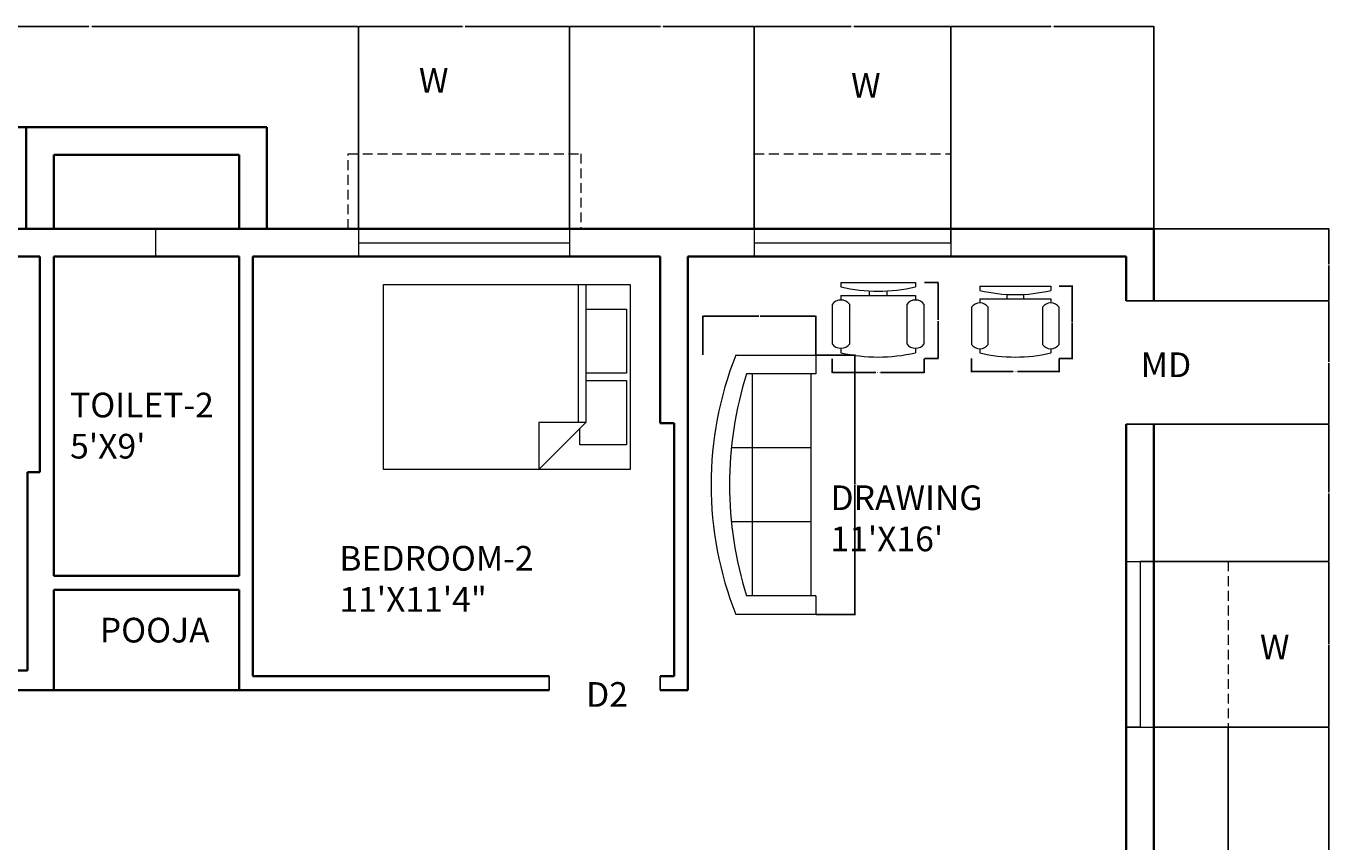
# Model space of a CAD drawing. Units: inches. Extents: x 514 to 1200, y -110 to 470.
# Tile 3 of 3: x 777 to 1200, y 206 to 470. Entities that reach past the tile are written whole.
import ezdxf

# ---------------------------------------------------------------- set-up
doc = ezdxf.new("R2010")
doc.units = ezdxf.units.IN
doc.linetypes.add('HIDDEN2', pattern=[4.7625, 3.175, -1.5875])
for name, color, linetype, lineweight in [('A-ANNO-DIMS', 2, 'Continuous', 18), ('A-ANNO-IDEN', 3, 'Continuous', 18), ('A-AREA-IDEN', 7, 'Continuous', 18), ('A-DOOR', 3, 'Continuous', 25), ('A-FLOR-OVHD', 8, 'HIDDEN2', 18), ('A-FURN', 8, 'Continuous', 18), ('A-GLAZ', 4, 'Continuous', 18), ('A-WALL', 7, 'Continuous', 35)]:
    doc.layers.add(name, color=color, linetype=linetype, lineweight=lineweight)
doc.dimstyles.get("Standard").update_dxf_attribs({"dimtxt": 0.18, "dimasz": 0.18, "dimexe": 0.18, "dimexo": 0.0625, "dimgap": 0.09, "dimtad": 0, "dimtih": 1, "dimtoh": 1, "dimdec": 4, "dimzin": 0, "dimdsep": 46, "dimtxsty": 'Standard', "dimcen": 0.09, "dimadec": 0, "dimazin": 0, "dimtfac": 1, "dimtdec": 4, "dimtofl": 0, "dimtmove": 0, "dimatfit": 3, "dimfxl": 1, "dimtolj": 1, "dimtzin": 0, "dimarcsym": 0})

# ---------------------------------------------------------------- blocks, each defined once
blk = doc.blocks.new('Chair - Desk')
for p, q in [((-8.5, 0), (-8.5, -1)), ((-8.5, 0), (8.5, 0)), ((8.5, 0), (8.5, -1)), ((-2, -3), (-2, -1.9355)), ((2, -1.9576), (2, -3)), ((-10.5, -5), (-10.5, -14)), ((-8.5, -3), (-8.5, -4)), ((-8.5, -3), (8.5, -3)), ((-6.5, -14), (-6.5, -5)), ((6.5, -5), (6.5, -14)), ((8.5, -3), (8.5, -4)), ((10.5, -14), (10.5, -5)), ((-8.5, -15), (-8.5, -16)), ((8.5, -15), (8.5, -16))]:
    blk.add_line(p, q)
for centre, radius, start, end in [((0, 34.625), 36.625, 256.5803, 283.4197), ((-8.5, -6.5), 2.5, 36.8699, 143.1301), ((8.5, -6.5), 2.5, 36.8699, 143.1301), ((-8.5, -12.5), 2.5, 216.8699, 323.1301), ((8.5, -12.5), 2.5, 216.8699, 323.1301), ((0, 19.625), 36.625, 256.5803, 283.4197)]:
    blk.add_arc(centre, radius, start, end)
blk = doc.blocks.new('Sofa - Roundback 7 ft.')
for p, q in [((-12.00002, -32.4421), (-12.00003, -6.5971)), ((11.99997, -32.4421), (11.99998, -6.5971)), ((-36.000027, -34), (-36.000027, -11.4696)), ((35.99998, -34), (35.99998, -11.4696)), ((-35.999844, -13.3819), (35.9998, -13.3819)), ((-36.000027, -32.4421), (35.99998, -32.4421))]:
    blk.add_line(p, q)
for points in [[(-36.000027, -34), (-42.000027, -34), (-42.000027, -8)], [(41.99998, -8), (41.99998, -34), (35.99998, -34)]]:
    blk.add_lwpolyline(points)
for centre, radius, start, end in [((0, -114.25), 114.25, 68.43141, 111.5686), ((-0.00001, -127.1968), 121.1968, 72.72033, 107.2797)]:
    blk.add_arc(centre, radius, start, end)
blk = doc.blocks.new('Bed - Queen')
for p, q in [((0, -80.00003), (0, 0)), ((0, 0), (59.99999, 0)), ((59.99999, 0), (59.99999, -80.00003)), ((7.99999, -1.2), (28.79998, -1.2)), ((7.99999, -14.4), (7.99999, -1.2)), ((28.79998, -1.2), (28.79998, -14.4)), ((31.19999, -1.2), (51.99999, -1.2)), ((31.19999, -14.4), (31.19999, -1.2)), ((51.99999, -1.2), (51.99999, -16.4)), ((0, -14.4), (44.8, -14.4)), ((44.8, -16.8), (0, -16.8)), ((59.99999, -29.6), (44.8, -14.4)), ((44.8, -14.4), (44.8, -29.6)), ((51.99999, -16.4), (46.79936, -16.4)), ((44.8, -29.6), (59.99999, -29.6)), ((59.99999, -80.00003), (0, -80.00003))]:
    blk.add_line(p, q)
blk = doc.blocks.new('WALL-BAY-60x24')
for p, q in [((0, 33), (0, 0)), ((9, 33), (9, 9)), ((69, 9), (69, 33)), ((78, 0), (78, 33)), ((9, 9), (69, 9)), ((0, 0), (78, 0))]:
    blk.add_line(p, q)
blk = doc.blocks.new('*D8')
at = {"layer": 'A-ANNO-DIMS', "color": 0, "lineweight": -2, "transparency": 16777216}
for p, q in [((1083.8, 362.46), (1083.8, 358.09)), ((1112.14, 362.46), (1112.14, 358.09)), ((1083.98, 358.27), (1097.22, 358.27)), ((1111.96, 358.27), (1098.72, 358.27))]:
    blk.add_line(p, q, dxfattribs=at)
at = {"layer": 'A-ANNO-DIMS', "color": 0, "transparency": 16777216}
for points in [[(1083.98, 358.3), (1083.98, 358.24), (1083.8, 358.27)], [(1111.96, 358.3), (1111.96, 358.24), (1112.14, 358.27)]]:
    blk.add_solid(points, dxfattribs=at)
at = {"layer": 'Defpoints', "color": 0, "transparency": 16777216}
for p in [(1083.8, 362.52), (1112.14, 362.52), (1112.14, 358.27)]:
    blk.add_point(p, dxfattribs=at)
at = {"layer": 'A-ANNO-DIMS', "color": 0, "transparency": 16777216, "insert": (1097.97, 358.27), "char_height": 0.18, "attachment_point": 5}
blk.add_mtext('\\A1;CHAIR 28', dxfattribs=at)
blk = doc.blocks.new('*D9')
at = {"layer": 'A-ANNO-DIMS', "color": 0, "lineweight": -2, "transparency": 16777216}
for p, q in [((1112.2, 385.91), (1116.57, 385.91)), ((1116.39, 385.73), (1116.39, 374.4)), ((1116.39, 362.7), (1116.39, 374.04)), ((1112.2, 362.52), (1116.57, 362.52))]:
    blk.add_line(p, q, dxfattribs=at)
at = {"layer": 'A-ANNO-DIMS', "color": 0, "transparency": 16777216}
for points in [[(1116.36, 385.73), (1116.42, 385.73), (1116.39, 385.91)], [(1116.36, 362.7), (1116.42, 362.7), (1116.39, 362.52)]]:
    blk.add_solid(points, dxfattribs=at)
at = {"layer": 'Defpoints', "color": 0, "transparency": 16777216}
for p in [(1112.14, 385.91), (1116.39, 385.91), (1112.14, 362.52)]:
    blk.add_point(p, dxfattribs=at)
at = {"layer": 'A-ANNO-DIMS', "color": 0, "transparency": 16777216, "insert": (1116.39, 374.22), "char_height": 0.18, "attachment_point": 5}
blk.add_mtext('\\A1;23', dxfattribs=at)
blk = doc.blocks.new('*D12')
at = {"layer": 'A-ANNO-DIMS', "color": 0, "lineweight": -2, "transparency": 16777216}
for p, q in [((1038.59, 362.44), (1038.59, 357.84)), ((1068.46, 362.44), (1068.46, 357.84)), ((1038.77, 358.02), (1052.79, 358.02)), ((1068.28, 358.02), (1054.26, 358.02))]:
    blk.add_line(p, q, dxfattribs=at)
at = {"layer": 'A-ANNO-DIMS', "color": 0, "transparency": 16777216}
for points in [[(1038.77, 358.05), (1038.77, 357.99), (1038.59, 358.02)], [(1068.28, 358.05), (1068.28, 357.99), (1068.46, 358.02)]]:
    blk.add_solid(points, dxfattribs=at)
at = {"layer": 'Defpoints', "color": 0, "transparency": 16777216}
for p in [(1038.59, 362.5), (1068.46, 362.5), (1068.46, 358.02)]:
    blk.add_point(p, dxfattribs=at)
at = {"layer": 'A-ANNO-DIMS', "color": 0, "transparency": 16777216, "insert": (1053.53, 358.02), "char_height": 0.18, "attachment_point": 5}
blk.add_mtext('\\A1;CHAIR 30', dxfattribs=at)
blk = doc.blocks.new('*D13')
at = {"layer": 'A-ANNO-DIMS', "color": 0, "lineweight": -2, "transparency": 16777216}
for p, q in [((1068.52, 387.15), (1073.12, 387.15)), ((1072.94, 386.97), (1072.94, 375.01)), ((1072.94, 362.68), (1072.94, 374.65)), ((1068.52, 362.5), (1073.12, 362.5))]:
    blk.add_line(p, q, dxfattribs=at)
at = {"layer": 'A-ANNO-DIMS', "color": 0, "transparency": 16777216}
for points in [[(1072.91, 386.97), (1072.97, 386.97), (1072.94, 387.15)], [(1072.91, 362.68), (1072.97, 362.68), (1072.94, 362.5)]]:
    blk.add_solid(points, dxfattribs=at)
at = {"layer": 'Defpoints', "color": 0, "transparency": 16777216}
for p in [(1068.46, 387.15), (1072.94, 387.15), (1068.46, 362.5)]:
    blk.add_point(p, dxfattribs=at)
at = {"layer": 'A-ANNO-DIMS', "color": 0, "transparency": 16777216, "insert": (1072.94, 374.83), "char_height": 0.18, "attachment_point": 5}
blk.add_mtext('\\A1;25', dxfattribs=at)
blk = doc.blocks.new('*D18')
at = {"layer": 'A-ANNO-DIMS', "color": 0, "lineweight": -2, "transparency": 16777216}
for p, q in [((1033.43, 363.59), (1046.15, 363.59)), ((1045.97, 363.41), (1045.97, 321.77)), ((1045.97, 279.77), (1045.97, 321.41)), ((1033.43, 279.59), (1046.15, 279.59))]:
    blk.add_line(p, q, dxfattribs=at)
at = {"layer": 'A-ANNO-DIMS', "color": 0, "transparency": 16777216}
for points in [[(1045.94, 363.41), (1046, 363.41), (1045.97, 363.59)], [(1045.94, 279.77), (1046, 279.77), (1045.97, 279.59)]]:
    blk.add_solid(points, dxfattribs=at)
at = {"layer": 'Defpoints', "color": 0, "transparency": 16777216}
for p in [(1033.37, 363.59), (1045.97, 363.59), (1033.37, 279.59)]:
    blk.add_point(p, dxfattribs=at)
at = {"layer": 'A-ANNO-DIMS', "color": 0, "transparency": 16777216, "insert": (1045.97, 321.59), "char_height": 0.18, "attachment_point": 5}
blk.add_mtext('\\A1;SOFA 84', dxfattribs=at)
blk = doc.blocks.new('*D19')
at = {"layer": 'A-ANNO-DIMS', "color": 0, "lineweight": -2, "transparency": 16777216}
for p, q in [((996.7, 363.65), (996.7, 376.37)), ((996.88, 376.19), (1014.8, 376.19)), ((1033.19, 376.19), (1015.28, 376.19)), ((1033.37, 363.65), (1033.37, 376.37))]:
    blk.add_line(p, q, dxfattribs=at)
at = {"layer": 'A-ANNO-DIMS', "color": 0, "transparency": 16777216}
for points in [[(996.88, 376.22), (996.88, 376.16), (996.7, 376.19)], [(1033.19, 376.22), (1033.19, 376.16), (1033.37, 376.19)]]:
    blk.add_solid(points, dxfattribs=at)
at = {"layer": 'Defpoints', "color": 0, "transparency": 16777216}
for p in [(996.7, 376.19), (996.7, 363.59), (1033.37, 363.59)]:
    blk.add_point(p, dxfattribs=at)
at = {"layer": 'A-ANNO-DIMS', "color": 0, "transparency": 16777216, "insert": (1015.04, 376.19), "char_height": 0.18, "attachment_point": 5}
blk.add_mtext('\\A1;37', dxfattribs=at)
blk = doc.blocks.new('*D26')
at = {"layer": 'A-ANNO-DIMS', "color": 0, "lineweight": -2, "transparency": 16777216}
for p, q in [((711.28, 404.58), (711.28, 470.25)), ((711.46, 470.07), (797.69, 470.07)), ((884.94, 470.07), (798.71, 470.07)), ((885.12, 404.58), (885.12, 470.25))]:
    blk.add_line(p, q, dxfattribs=at)
at = {"layer": 'A-ANNO-DIMS', "color": 0, "transparency": 16777216}
for points in [[(711.46, 470.1), (711.46, 470.04), (711.28, 470.07)], [(884.94, 470.1), (884.94, 470.04), (885.12, 470.07)]]:
    blk.add_solid(points, dxfattribs=at)
at = {"layer": 'Defpoints', "color": 0, "transparency": 16777216}
for p in [(885.12, 470.07), (711.28, 404.52), (885.12, 404.52)]:
    blk.add_point(p, dxfattribs=at)
at = {"layer": 'A-ANNO-DIMS', "color": 0, "transparency": 16777216, "insert": (798.2, 470.07), "char_height": 0.18, "attachment_point": 5}
blk.add_mtext('\\A1;173.83', dxfattribs=at)
blk = doc.blocks.new('*D27')
at = {"layer": 'A-ANNO-DIMS', "color": 0, "lineweight": -2, "transparency": 16777216}
for p, q in [((885.12, 404.58), (885.12, 470.25)), ((885.3, 470.07), (918.83, 470.07)), ((953.26, 470.07), (919.73, 470.07)), ((953.44, 404.58), (953.44, 470.25))]:
    blk.add_line(p, q, dxfattribs=at)
at = {"layer": 'A-ANNO-DIMS', "color": 0, "transparency": 16777216}
for points in [[(885.3, 470.1), (885.3, 470.04), (885.12, 470.07)], [(953.26, 470.1), (953.26, 470.04), (953.44, 470.07)]]:
    blk.add_solid(points, dxfattribs=at)
at = {"layer": 'Defpoints', "color": 0, "transparency": 16777216}
for p in [(953.44, 470.07), (885.12, 404.52), (953.44, 404.52)]:
    blk.add_point(p, dxfattribs=at)
at = {"layer": 'A-ANNO-DIMS', "color": 0, "transparency": 16777216, "insert": (919.28, 470.07), "char_height": 0.18, "attachment_point": 5}
blk.add_mtext('\\A1;68.32', dxfattribs=at)
blk = doc.blocks.new('*D28')
at = {"layer": 'A-ANNO-DIMS', "color": 0, "lineweight": -2, "transparency": 16777216}
for p, q in [((953.44, 404.58), (953.44, 470.25)), ((953.62, 470.07), (982.96, 470.07)), ((1013.2, 470.07), (983.86, 470.07)), ((1013.38, 404.58), (1013.38, 470.25))]:
    blk.add_line(p, q, dxfattribs=at)
at = {"layer": 'A-ANNO-DIMS', "color": 0, "transparency": 16777216}
for points in [[(953.62, 470.1), (953.62, 470.04), (953.44, 470.07)], [(1013.2, 470.1), (1013.2, 470.04), (1013.38, 470.07)]]:
    blk.add_solid(points, dxfattribs=at)
at = {"layer": 'Defpoints', "color": 0, "transparency": 16777216}
for p in [(1013.38, 470.07), (953.44, 404.52), (1013.38, 404.52)]:
    blk.add_point(p, dxfattribs=at)
at = {"layer": 'A-ANNO-DIMS', "color": 0, "transparency": 16777216, "insert": (983.41, 470.07), "char_height": 0.18, "attachment_point": 5}
blk.add_mtext('\\A1;59.94', dxfattribs=at)
blk = doc.blocks.new('*D29')
at = {"layer": 'A-ANNO-DIMS', "color": 0, "lineweight": -2, "transparency": 16777216}
for p, q in [((1013.377732, 404.583196), (1013.377732, 470.250696)), ((1013.557732, 470.070696), (1044.750738, 470.070696)), ((1076.843744, 470.070696), (1045.650738, 470.070696)), ((1077.023744, 404.583196), (1077.023744, 470.250696))]:
    blk.add_line(p, q, dxfattribs=at)
at = {"layer": 'A-ANNO-DIMS', "color": 0, "transparency": 16777216}
for points in [[(1013.557732, 470.100696), (1013.557732, 470.040696), (1013.377732, 470.070696)], [(1076.843744, 470.100696), (1076.843744, 470.040696), (1077.023744, 470.070696)]]:
    blk.add_solid(points, dxfattribs=at)
at = {"layer": 'Defpoints', "color": 0, "transparency": 16777216}
for p in [(1077.023744, 470.070696), (1013.377732, 404.520696), (1077.023744, 404.520696)]:
    blk.add_point(p, dxfattribs=at)
at = {"layer": 'A-ANNO-DIMS', "color": 0, "transparency": 16777216, "insert": (1045.200738, 470.070696), "char_height": 0.18, "attachment_point": 5}
blk.add_mtext('\\A1;63.65', dxfattribs=at)
blk = doc.blocks.new('*D30')
at = {"layer": 'A-ANNO-DIMS', "color": 0, "lineweight": -2, "transparency": 16777216}
for p, q in [((1077.023744, 404.583196), (1077.023744, 470.250696)), ((1077.203744, 470.070696), (1109.507154, 470.070696)), ((1142.710564, 470.070696), (1110.407154, 470.070696)), ((1142.890564, 404.583196), (1142.890564, 470.250696))]:
    blk.add_line(p, q, dxfattribs=at)
at = {"layer": 'A-ANNO-DIMS', "color": 0, "transparency": 16777216}
for points in [[(1077.203744, 470.100696), (1077.203744, 470.040696), (1077.023744, 470.070696)], [(1142.710564, 470.100696), (1142.710564, 470.040696), (1142.890564, 470.070696)]]:
    blk.add_solid(points, dxfattribs=at)
at = {"layer": 'Defpoints', "color": 0, "transparency": 16777216}
for p in [(1142.890564, 470.070696), (1077.023744, 404.520696), (1142.890564, 404.520696)]:
    blk.add_point(p, dxfattribs=at)
at = {"layer": 'A-ANNO-DIMS', "color": 0, "transparency": 16777216, "insert": (1109.957154, 470.070696), "char_height": 0.18, "attachment_point": 5}
blk.add_mtext('\\A1;65.87', dxfattribs=at)
blk = doc.blocks.new('*D31')
at = {"layer": 'A-ANNO-DIMS', "color": 0, "lineweight": -2, "transparency": 16777216}
for p, q in [((1142.953064, 404.520696), (1199.719295, 404.520696)), ((1199.539295, 404.340696), (1199.539295, 393.046922)), ((1199.539295, 381.393148), (1199.539295, 392.686922)), ((1142.953064, 381.213148), (1199.719295, 381.213148))]:
    blk.add_line(p, q, dxfattribs=at)
at = {"layer": 'A-ANNO-DIMS', "color": 0, "transparency": 16777216}
for points in [[(1199.509295, 404.340696), (1199.569295, 404.340696), (1199.539295, 404.520696)], [(1199.509295, 381.393148), (1199.569295, 381.393148), (1199.539295, 381.213148)]]:
    blk.add_solid(points, dxfattribs=at)
at = {"layer": 'Defpoints', "color": 0, "transparency": 16777216}
for p in [(1142.890564, 404.520696), (1142.890564, 381.213148), (1199.539295, 381.213148)]:
    blk.add_point(p, dxfattribs=at)
at = {"layer": 'A-ANNO-DIMS', "color": 0, "transparency": 16777216, "insert": (1199.539295, 392.866922), "char_height": 0.18, "attachment_point": 5}
blk.add_mtext('\\A1;23.308', dxfattribs=at)
blk = doc.blocks.new('*D32')
at = {"layer": 'A-ANNO-DIMS', "color": 0, "lineweight": -2, "transparency": 16777216}
for p, q in [((1142.953064, 381.213148), (1199.719295, 381.213148)), ((1199.539295, 381.033148), (1199.539295, 361.393148)), ((1199.539295, 341.393148), (1199.539295, 361.033148)), ((1142.953064, 341.213148), (1199.719295, 341.213148))]:
    blk.add_line(p, q, dxfattribs=at)
at = {"layer": 'A-ANNO-DIMS', "color": 0, "transparency": 16777216}
for points in [[(1199.509295, 381.033148), (1199.569295, 381.033148), (1199.539295, 381.213148)], [(1199.509295, 341.393148), (1199.569295, 341.393148), (1199.539295, 341.213148)]]:
    blk.add_solid(points, dxfattribs=at)
at = {"layer": 'Defpoints', "color": 0, "transparency": 16777216}
for p in [(1142.890564, 381.213148), (1142.890564, 341.213148), (1199.539295, 341.213148)]:
    blk.add_point(p, dxfattribs=at)
at = {"layer": 'A-ANNO-DIMS', "color": 0, "transparency": 16777216, "insert": (1199.539295, 361.213148), "char_height": 0.18, "attachment_point": 5}
blk.add_mtext('\\A1;40', dxfattribs=at)
blk = doc.blocks.new('*D33')
at = {"layer": 'A-ANNO-DIMS', "color": 0, "lineweight": -2, "transparency": 16777216}
for p, q in [((1142.953064, 341.213148), (1199.719295, 341.213148)), ((1199.539295, 341.033148), (1199.539295, 319.140993)), ((1199.539295, 296.888838), (1199.539295, 318.780993)), ((1142.953064, 296.708838), (1199.719295, 296.708838))]:
    blk.add_line(p, q, dxfattribs=at)
at = {"layer": 'A-ANNO-DIMS', "color": 0, "transparency": 16777216}
for points in [[(1199.509295, 341.033148), (1199.569295, 341.033148), (1199.539295, 341.213148)], [(1199.509295, 296.888838), (1199.569295, 296.888838), (1199.539295, 296.708838)]]:
    blk.add_solid(points, dxfattribs=at)
at = {"layer": 'Defpoints', "color": 0, "transparency": 16777216}
for p in [(1142.890564, 341.213148), (1142.890564, 296.708838), (1199.539295, 296.708838)]:
    blk.add_point(p, dxfattribs=at)
at = {"layer": 'A-ANNO-DIMS', "color": 0, "transparency": 16777216, "insert": (1199.539295, 318.960993), "char_height": 0.18, "attachment_point": 5}
blk.add_mtext('\\A1;44.5', dxfattribs=at)
blk = doc.blocks.new('*D34')
at = {"layer": 'A-ANNO-DIMS', "color": 0, "lineweight": -2, "transparency": 16777216}
for p, q in [((1142.953064, 296.708838), (1199.719295, 296.708838)), ((1199.539295, 296.528838), (1199.539295, 270.069776)), ((1199.539295, 243.250714), (1199.539295, 269.709776)), ((1142.953064, 243.070714), (1199.719295, 243.070714))]:
    blk.add_line(p, q, dxfattribs=at)
at = {"layer": 'A-ANNO-DIMS', "color": 0, "transparency": 16777216}
for points in [[(1199.509295, 296.528838), (1199.569295, 296.528838), (1199.539295, 296.708838)], [(1199.509295, 243.250714), (1199.569295, 243.250714), (1199.539295, 243.070714)]]:
    blk.add_solid(points, dxfattribs=at)
at = {"layer": 'Defpoints', "color": 0, "transparency": 16777216}
for p in [(1142.890564, 296.708838), (1142.890564, 243.070714), (1199.539295, 243.070714)]:
    blk.add_point(p, dxfattribs=at)
at = {"layer": 'A-ANNO-DIMS', "color": 0, "transparency": 16777216, "insert": (1199.539295, 269.889776), "char_height": 0.18, "attachment_point": 5}
blk.add_mtext('\\A1;53.64', dxfattribs=at)
blk = doc.blocks.new('*D35')
at = {"layer": 'A-ANNO-DIMS', "color": 0, "lineweight": -2, "transparency": 16777216}
for p, q in [((1142.953064, 243.070714), (1199.719295, 243.070714)), ((1199.539295, 242.890714), (1199.539295, 136.225705)), ((1199.539295, 29.200696), (1199.539295, 135.865705)), ((1142.953064, 29.020696), (1199.719295, 29.020696))]:
    blk.add_line(p, q, dxfattribs=at)
at = {"layer": 'A-ANNO-DIMS', "color": 0, "transparency": 16777216}
for points in [[(1199.509295, 242.890714), (1199.569295, 242.890714), (1199.539295, 243.070714)], [(1199.509295, 29.200696), (1199.569295, 29.200696), (1199.539295, 29.020696)]]:
    blk.add_solid(points, dxfattribs=at)
at = {"layer": 'Defpoints', "color": 0, "transparency": 16777216}
for p in [(1142.890564, 243.070714), (1142.890564, 29.020696), (1199.539295, 29.020696)]:
    blk.add_point(p, dxfattribs=at)
at = {"layer": 'A-ANNO-DIMS', "color": 0, "transparency": 16777216, "insert": (1199.539295, 136.045705), "char_height": 0.18, "attachment_point": 5}
blk.add_mtext('\\A1;214.05', dxfattribs=at)
blk = doc.blocks.new('*D36')
at = {"layer": 'A-ANNO-DIMS', "color": 0, "lineweight": -2, "transparency": 16777216}
for p, q in [((1166.99, 243.01), (1166.99, -83.71)), ((547.32, 185.96), (547.32, -83.71)), ((547.5, -83.53), (856.73, -83.53)), ((1166.81, -83.53), (857.57, -83.53))]:
    blk.add_line(p, q, dxfattribs=at)
at = {"layer": 'A-ANNO-DIMS', "color": 0, "transparency": 16777216}
for points in [[(547.5, -83.5), (547.5, -83.56), (547.32, -83.53)], [(1166.81, -83.5), (1166.81, -83.56), (1166.99, -83.53)]]:
    blk.add_solid(points, dxfattribs=at)
at = {"layer": 'Defpoints', "color": 0, "transparency": 16777216}
for p in [(1166.99, 243.07), (547.32, 186.02), (1166.99, -83.53)]:
    blk.add_point(p, dxfattribs=at)
at = {"layer": 'A-ANNO-DIMS', "color": 0, "transparency": 16777216, "insert": (857.15, -83.53), "char_height": 0.18, "attachment_point": 5}
blk.add_mtext('\\A1;619.7', dxfattribs=at)
blk = doc.blocks.new('*D37')
at = {"layer": 'A-ANNO-DIMS', "color": 0, "lineweight": -2, "transparency": 16777216}
for p, q in [((719.82324, 437.520696), (514.588716, 437.520696)), ((514.768716, 437.340696), (514.768716, 193.450696)), ((514.768716, -50.799304), (514.768716, 193.090696)), ((846.828064, -50.979304), (514.588716, -50.979304))]:
    blk.add_line(p, q, dxfattribs=at)
at = {"layer": 'A-ANNO-DIMS', "color": 0, "transparency": 16777216}
for points in [[(514.738716, 437.340696), (514.798716, 437.340696), (514.768716, 437.520696)], [(514.738716, -50.799304), (514.798716, -50.799304), (514.768716, -50.979304)]]:
    blk.add_solid(points, dxfattribs=at)
at = {"layer": 'Defpoints', "color": 0, "transparency": 16777216}
for p in [(514.768716, 437.520696), (719.88574, 437.520696), (846.890564, -50.979304)]:
    blk.add_point(p, dxfattribs=at)
at = {"layer": 'A-ANNO-DIMS', "color": 0, "transparency": 16777216, "insert": (514.768716, 193.270696), "char_height": 0.18, "attachment_point": 5}
blk.add_mtext('\\A1;488.5', dxfattribs=at)

msp = doc.modelspace()

# ---------------------------------------------------------------- linework, layer by layer
at = {"layer": 'A-DOOR'}
for p, q in [((1133.8906, 381.2131), (1142.8906, 381.2131)), ((1142.8906, 341.2131), (1133.8906, 341.2131)), ((1138.3906, 341.2131), (1142.8906, 341.2131)), ((946.8906, 255.0207), (946.8906, 259.5207)), ((982.8906, 255.0207), (982.8906, 259.5207))]:
    msp.add_line(p, q, dxfattribs=at)
at = {"layer": 'A-FLOR-OVHD'}
for p, q in [((881.7608, 404.5207), (881.7608, 428.8855)), ((881.7608, 428.8855), (957.1619, 428.8855)), ((957.1619, 428.8855), (957.1619, 404.5207)), ((1013.3777, 404.5207), (1013.3777, 428.8855)), ((1013.3777, 428.8855), (1077.0237, 428.8855)), ((1077.0237, 428.8855), (1077.0237, 404.5207)), ((1142.8906, 296.7088), (1166.9893, 296.7088)), ((1166.9893, 296.7088), (1166.9893, 243.0707)), ((1166.9893, 243.0707), (1142.8906, 243.0707))]:
    msp.add_line(p, q, dxfattribs=at)
at = {"layer": 'A-GLAZ'}
for p, q in [((819.3159, 404.5207), (819.3159, 395.5207)), ((885.1179, 404.5207), (885.1179, 395.5207)), ((953.4385, 404.5207), (953.4385, 395.5207)), ((1013.3777, 404.5207), (1013.3777, 395.5207)), ((1077.0237, 404.5207), (1077.0237, 395.5207)), ((1077.0237, 400.0207), (1077.0237, 404.5207)), ((1077.0237, 404.5207), (1077.0237, 395.5207)), ((885.1179, 400.0207), (953.4385, 400.0207)), ((1013.3777, 400.0207), (1077.0237, 400.0207)), ((1133.8906, 296.7088), (1142.8906, 296.7088)), ((1142.8906, 296.7088), (1138.3906, 296.7088)), ((1138.3906, 296.7088), (1138.3906, 243.0707)), ((1138.3906, 243.0707), (1133.8906, 243.0707)), ((1133.8906, 243.0707), (1142.8906, 243.0707))]:
    msp.add_line(p, q, dxfattribs=at)
at = {"layer": 'A-WALL'}
for p, q in [((777.3906, 437.5207), (728.8857, 437.5207)), ((728.8857, 404.5207), (1142.8906, 404.5207)), ((1142.8906, 395.5207), (1142.8906, 404.5207)), ((609.8906, 395.5207), (781.8906, 395.5207)), ((781.8906, 325.6278), (781.8906, 395.5207)), ((786.3906, 292.0207), (786.3906, 395.5207)), ((786.3906, 395.5207), (846.3906, 395.5207)), ((846.3906, 292.0207), (846.3906, 395.5207)), ((850.8906, 259.5207), (850.8906, 395.5207)), ((850.8906, 395.5207), (982.8906, 395.5207)), ((982.8906, 341.5561), (982.8906, 395.5207)), ((991.8906, 255.0207), (991.8906, 395.5207)), ((991.8906, 395.5207), (1133.8906, 395.5207)), ((1133.8906, 381.2131), (1133.8906, 395.5207)), ((1142.8906, 381.2131), (1142.8906, 395.5207)), ((982.8906, 341.5561), (987.3906, 341.5561)), ((987.3906, 259.5207), (987.3906, 341.5561)), ((1133.8906, 255.0207), (1133.8906, 341.2131)), ((1142.8906, 255.0207), (1142.8906, 341.2131)), ((777.8906, 261.4252), (777.8906, 325.6278)), ((777.8906, 325.6278), (781.8906, 325.6278)), ((786.3906, 292.0207), (846.3906, 292.0207)), ((786.3906, 255.0207), (786.3906, 287.5207)), ((786.3906, 287.5207), (846.3906, 287.5207)), ((846.3906, 255.0207), (846.3906, 287.5207)), ((772.9065, 261.4252), (777.8906, 261.4252)), ((850.8906, 259.5207), (946.8906, 259.5207)), ((987.3906, 259.5207), (982.8906, 259.5207)), ((777.8906, 255.0207), (772.9065, 255.0207)), ((777.8906, 255.0207), (786.3906, 255.0207)), ((777.8906, 255.0207), (946.8906, 255.0207)), ((786.3906, 255.0207), (846.3906, 255.0207)), ((991.8906, 255.0207), (982.8906, 255.0207)), ((1133.8906, 255.0207), (1133.8906, 199.0207)), ((1142.8906, 255.0207), (1142.8906, 199.0207))]:
    msp.add_line(p, q, dxfattribs=at)

# ---------------------------------------------------------------- block references
at = {"layer": 'A-FURN'}
for name, p, rotation in [('Bed - Queen', (973.1991, 386.5264), 270), ('Sofa - Roundback 7 ft.', (999.3688, 321.5877), 90)]:
    msp.add_blockref(name, p, dxfattribs=dict(at, rotation=rotation))
for p, xscale, yscale, zscale in [((1053.5268, 387.1502), 1.422102317285446, 1.422102317285446, 1.422102317285446), ((1097.9695, 385.9114), 1.349230775328343, 1.349230775328343, 1.349230775328343)]:
    msp.add_blockref('Chair - Desk', p, dxfattribs=dict(at, xscale=xscale, yscale=yscale, zscale=zscale))
at = {"layer": 'A-WALL', "rotation": 180}
msp.add_blockref('WALL-BAY-60x24', (855.3906, 437.5207), dxfattribs=at)

# ---------------------------------------------------------------- texts
at = {"layer": 'A-ANNO-IDEN', "char_height": 8, "attachment_point": 1}
for s, insert in [('{\\fTimes New Roman|b0|i0|c0|p18;W}', (904.6938, 456.6502)), ('{\\fTimes New Roman|b0|i0|c0|p18;W}', (1044.7366, 455.055)), ('{\\fTimes New Roman|b0|i0|c0|p18;MD}', (1138.598, 364.4832)), ('{\\fTimes New Roman|b0|i0|c0|p18;W}', (1177.2378, 273.0239)), ('{\\fTimes New Roman|b0|i0|c0|p18;D2}', (958.8675, 257.6241))]:
    msp.add_mtext_dynamic_manual_height_columns(s, width=92.773282, gutter_width=12.5, heights=[0], dxfattribs=dict(at, insert=insert))
at = {"layer": 'A-AREA-IDEN', "char_height": 8, "attachment_point": 1}
for s, insert in [("{\\fTimes New Roman|b0|i0|c0|p18;TOILET-2\\P5'X9'}", (791.661, 351.4229)), ("{\\fTimes New Roman|b0|i0|c0|p18;DRAWING\\P11'X16'}", (1038.0527, 321.3746)), ('{\\fTimes New Roman|b0|i0|c0|p18;BEDROOM-2\\P11\'X11\'4"}', (878.9146, 301.7593)), ('{\\fTimes New Roman|b0|i0|c0|p18;POOJA}', (801.2933, 278.4627))]:
    msp.add_mtext_dynamic_manual_height_columns(s, width=92.773282, gutter_width=12.5, heights=[0], dxfattribs=dict(at, insert=insert))

# ---------------------------------------------------------------- dimensions: what is measured, and where the dimension line sits
at = {"layer": 'A-ANNO-DIMS'}
for base, p1, p2, override, picture, middle in [((885.1179, 470.0707), (711.283, 404.5207), (885.1179, 404.5207), {"dimdec": 2, "dimlfac": 1, "dimrnd": 0, "dimzin": 0, "dimdsep": 46, "dimlunit": 2}, '*D26', (798.2005, 470.0707)), ((953.4385, 470.0707), (885.1179, 404.5207), (953.4385, 404.5207), {"dimdec": 2, "dimlfac": 1, "dimrnd": 0, "dimzin": 0, "dimdsep": 46, "dimlunit": 2}, '*D27', (919.2782, 470.0707)), ((1013.3777, 470.0707), (953.4385, 404.5207), (1013.3777, 404.5207), {"dimdec": 2, "dimlfac": 1, "dimrnd": 0, "dimzin": 0, "dimdsep": 46, "dimlunit": 2}, '*D28', (983.4081, 470.0707)), ((1077.0237, 470.0707), (1013.3777, 404.5207), (1077.0237, 404.5207), {"dimdec": 2, "dimlfac": 1, "dimrnd": 0, "dimzin": 0, "dimdsep": 46, "dimlunit": 2}, '*D29', (1045.2007, 470.0707)), ((1142.8906, 470.0707), (1077.0237, 404.5207), (1142.8906, 404.5207), {"dimdec": 2, "dimlfac": 1, "dimrnd": 0, "dimzin": 0, "dimdsep": 46, "dimlunit": 2}, '*D30', (1109.9572, 470.0707)), ((1166.9893, -83.5293), (547.3187, 186.0207), (1166.9893, 243.0707), {"dimdec": 1, "dimlfac": 1, "dimrnd": 0, "dimzin": 0, "dimdsep": 46, "dimlunit": 2}, '*D36', (857.154, -83.5293))]:
    dim = msp.add_linear_dim(base=base, p1=p1, p2=p2, dimstyle='Standard', override=override, dxfattribs=at)
    dim.commit()
    dim.dimension.update_dxf_attribs({"geometry": picture, "text_midpoint": middle})
for base, p1, p2, angle, override, picture, middle in [((514.7687, 437.5207), (846.8906, -50.9793), (719.8857, 437.5207), 90, {"dimdec": 1, "dimlfac": 1, "dimrnd": 0, "dimzin": 0, "dimdsep": 46, "dimlunit": 2}, '*D37', (514.7687, 193.2707)), ((1199.5393, 381.2131), (1142.8906, 404.5207), (1142.8906, 381.2131), 90, {"dimdec": 3, "dimlfac": 1, "dimrnd": 0, "dimzin": 0, "dimdsep": 46, "dimlunit": 2}, '*D31', (1199.5393, 392.8669)), ((1072.9385, 387.1502), (1068.4589, 362.5004), (1068.4589, 387.1502), 90, {"dimdec": 0, "dimlfac": 1, "dimrnd": 0, "dimzin": 0, "dimdsep": 46, "dimlunit": 2}, '*D13', (1072.9385, 374.8253)), ((1116.3865, 385.9114), (1112.1364, 362.5247), (1112.1364, 385.9114), 90, {"dimdec": 0, "dimlfac": 1, "dimrnd": 0, "dimzin": 0, "dimdsep": 46, "dimlunit": 2}, '*D9', (1116.3865, 374.2181)), ((1199.5393, 341.2131), (1142.8906, 381.2131), (1142.8906, 341.2131), 90, {"dimdec": 0, "dimlfac": 1, "dimrnd": 0, "dimzin": 0, "dimdsep": 46, "dimlunit": 2}, '*D32', (1199.5393, 361.2131)), ((996.7022, 376.1877), (1033.3688, 363.5877), (996.7022, 363.5877), 180, {"dimdec": 0, "dimlfac": 1, "dimrnd": 0, "dimzin": 0, "dimdsep": 46, "dimlunit": 2}, '*D19', (1015.0355, 376.1877)), ((1199.5393, 296.7088), (1142.8906, 341.2131), (1142.8906, 296.7088), 90, {"dimdec": 1, "dimlfac": 1, "dimrnd": 0, "dimzin": 0, "dimdsep": 46, "dimlunit": 2}, '*D33', (1199.5393, 318.961)), ((1199.5393, 243.0707), (1142.8906, 296.7088), (1142.8906, 243.0707), 90, {"dimdec": 2, "dimlfac": 1, "dimrnd": 0, "dimzin": 0, "dimdsep": 46, "dimlunit": 2}, '*D34', (1199.5393, 269.8898)), ((1199.5393, 29.0207), (1142.8906, 243.0707), (1142.8906, 29.0207), 90, {"dimdec": 2, "dimlfac": 1, "dimrnd": 0, "dimzin": 0, "dimdsep": 46, "dimlunit": 2}, '*D35', (1199.5393, 136.0457))]:
    dim = msp.add_linear_dim(base=base, p1=p1, p2=p2, angle=angle, dimstyle='Standard', override=override, dxfattribs=at)
    dim.commit()
    dim.dimension.update_dxf_attribs({"geometry": picture, "text_midpoint": middle})
dim = msp.add_linear_dim(base=(1045.9688, 363.5877), p1=(1033.3688, 279.5877), p2=(1033.3688, 363.5877), angle=90, text='SOFA <>', dimstyle='Standard', override={"dimdec": 0, "dimlfac": 1, "dimrnd": 0, "dimzin": 0, "dimdsep": 46, "dimlunit": 2}, dxfattribs=at)
dim.commit()
dim.dimension.update_dxf_attribs({"geometry": '*D18', "text_midpoint": (1045.9688, 321.5877)})
for base, p1, p2, picture, middle in [((1068.4589, 358.0208), (1038.5947, 362.5004), (1068.4589, 362.5004), '*D12', (1053.5268, 358.0208)), ((1112.1364, 358.2746), (1083.8026, 362.5247), (1112.1364, 362.5247), '*D8', (1097.9695, 358.2746))]:
    dim = msp.add_linear_dim(base=base, p1=p1, p2=p2, text='CHAIR <>', dimstyle='Standard', override={"dimdec": 0, "dimlfac": 1, "dimrnd": 0, "dimzin": 0, "dimdsep": 46, "dimlunit": 2}, dxfattribs=at)
    dim.commit()
    dim.dimension.update_dxf_attribs({"geometry": picture, "text_midpoint": middle})

doc.saveas('drawing.dxf')
